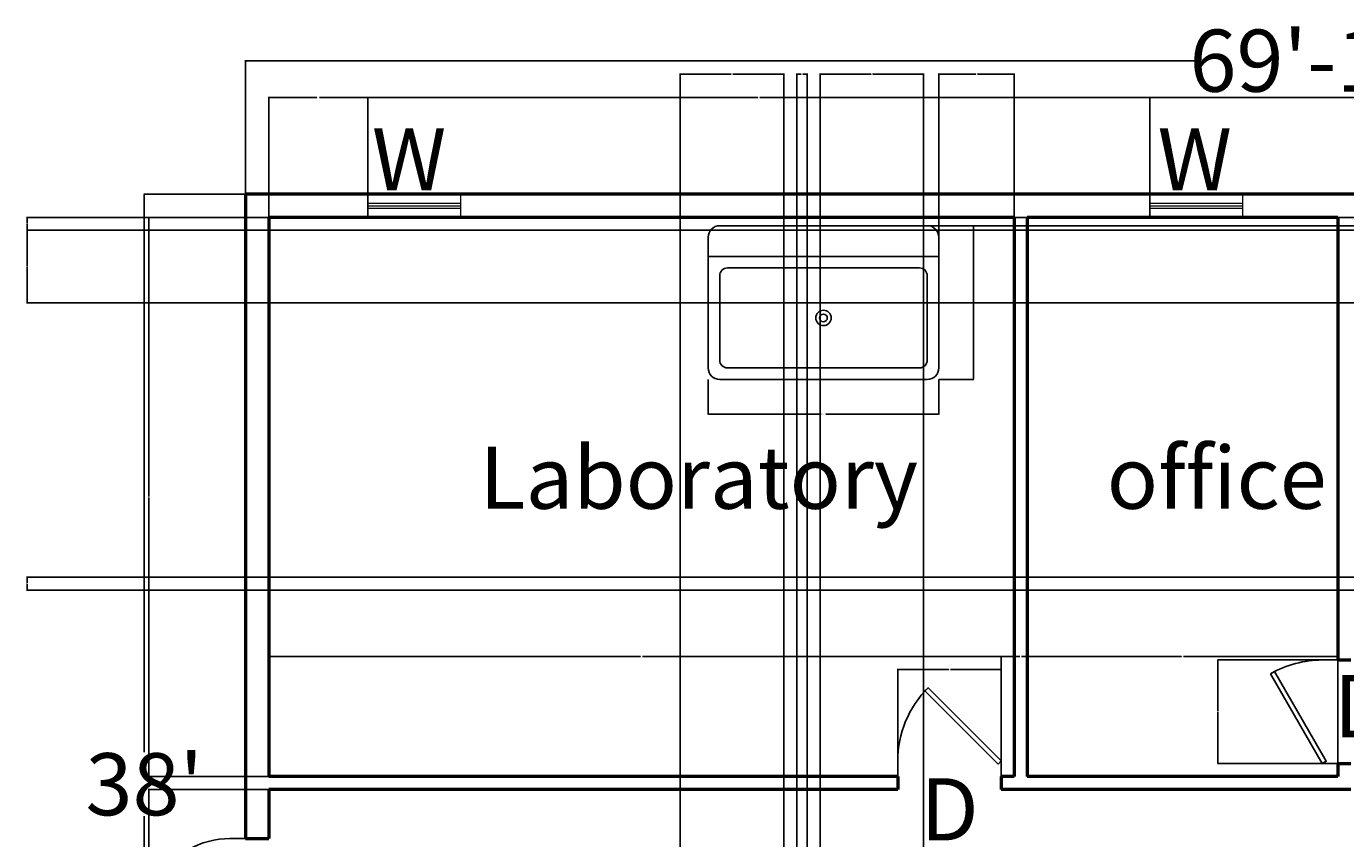
# Model space of a CAD drawing. Units: inches. Extents: x -84 to 931, y 65 to 668.
# Tile 2 of 5: x -84 to 426, y 355 to 668. Entities that reach past the tile are written whole.
import ezdxf

# ---------------------------------------------------------------- set-up
doc = ezdxf.new("R2010")
doc.units = ezdxf.units.IN
doc.header["$MEASUREMENT"] = 0
for name, color, linetype, lineweight in [('A-ANNO-DIMS', 2, 'Continuous', 18), ('A-ANNO-TEXT', 7, 'Continuous', 18), ('A-AREA-IDEN', 7, 'Continuous', 25), ('A-DOOR', 4, 'Continuous', 25), ('A-FLOR-FIXT', 9, 'Continuous', 25), ('A-GLAZ', 4, 'Continuous', 18), ('A-WALL', 7, 'Continuous', 50)]:
    doc.layers.add(name, color=color, linetype=linetype, lineweight=lineweight)
doc.styles.get("Standard").update_dxf_attribs({"font": 'arial.ttf'})
doc.dimstyles.get("Standard").update_dxf_attribs({"dimtxt": 0.18, "dimasz": 0.18, "dimexe": 0.18, "dimexo": 0.0625, "dimgap": 0.09, "dimtad": 0, "dimtih": 1, "dimtoh": 1, "dimdec": 0, "dimzin": 0, "dimdsep": 46, "dimlunit": 3, "dimtxsty": 'Standard', "dimcen": 0.09, "dimadec": 0, "dimazin": 0, "dimtfac": 1, "dimtdec": 0, "dimtofl": 0, "dimtmove": 0, "dimatfit": 3, "dimfxl": 1, "dimtolj": 1, "dimtzin": 0, "dimarcsym": 0})

# ---------------------------------------------------------------- blocks, each defined once
blk = doc.blocks.new('*U2')
for p, q in [((0, 0), (0, -6)), ((-40, 0), (-40, -6))]:
    blk.add_line(p, q)
blk.add_lwpolyline([(0, 0), (-28.28, 28.28), (-29.52, 27.05), (-1.24, -1.24)], close=True)
blk.add_arc((0, 0), 40, 135, 180)
blk = doc.blocks.new('*U3')
for p, q in [((0, 0), (0, -6)), ((40, 0), (40, -6))]:
    blk.add_line(p, q)
blk.add_lwpolyline([(0, 0), (34.64, 20), (35.52, 18.48), (0.88, -1.52)], close=True)
blk.add_arc((0, 0), 40, 0, 30)
blk = doc.blocks.new('*U11')
for p, q in [((0, 0), (0, -6)), ((32, 0), (32, -6))]:
    blk.add_line(p, q)
blk.add_lwpolyline([(0, 0), (27.71, 16), (28.59, 14.48), (0.87, -1.52)], close=True)
blk.add_arc((0, 0), 32, 0, 30)
blk = doc.blocks.new('Sink-single - 30 in top')
blk.add_line((-15, -3.999996), (15, -3.999996))
for points in [[(-13.5, 0), (13.5, 0)], [(-15, -18.499996), (-15, -1.5)], [(15, -1.5), (15, -18.499996)], [(-13.5, -17.499996), (-13.5, -6.499996)], [(-12.5, -5.499996), (12.5, -5.499996)], [(13.5, -6.499996), (13.5, -17.499996)], [(12.5, -18.499996), (-12.5, -18.499996)], [(13.5, -19.999996), (-13.5, -19.999996)]]:
    blk.add_lwpolyline(points)
for radius in [1, 0.5]:
    blk.add_circle((0, -11.999996), radius)
for centre, radius, start, end in [((-13.5, -1.5), 1.5, 90, 180), ((13.5, -1.5), 1.5, 0, 90), ((-12.5, -6.499996), 1, 90, 180), ((12.5, -6.499996), 1, 0, 90), ((-13.5, -18.499996), 1.5, 180, 270), ((-12.5, -17.499996), 1, 180, 270), ((12.5, -17.499996), 1, 270, 0), ((13.5, -18.499996), 1.5, 270, 0)]:
    blk.add_arc(centre, radius, start, end)
blk = doc.blocks.new('*D17')
at = {"layer": 'A-ANNO-DIMS', "color": 0, "lineweight": -2, "transparency": 16777216}
for p, q in [((0.53, 603.58), (0.53, 655.22)), ((0.71, 655.04), (368.83, 655.04)), ((838.35, 655.04), (470.23, 655.04)), ((838.53, 603.58), (838.53, 655.22))]:
    blk.add_line(p, q, dxfattribs=at)
at = {"layer": 'A-ANNO-DIMS', "color": 0, "transparency": 16777216}
for points in [[(0.71, 655.07), (0.71, 655.01), (0.53, 655.04)], [(838.35, 655.07), (838.35, 655.01), (838.53, 655.04)]]:
    blk.add_solid(points, dxfattribs=at)
at = {"layer": 'Defpoints', "color": 0, "transparency": 16777216}
for p in [(838.53, 655.04), (0.53, 603.52), (838.53, 603.52)]:
    blk.add_point(p, dxfattribs=at)
at = {"layer": 'A-ANNO-DIMS', "color": 0, "transparency": 16777216, "insert": (419.53, 655.04), "char_height": 0.18, "attachment_point": 5}
blk.add_mtext('\\A1;{\\H133.33333x;69\'-10"}', dxfattribs=at)
blk = doc.blocks.new('*D18')
at = {"layer": 'A-ANNO-DIMS', "color": 0, "lineweight": -2, "transparency": 16777216}
for p, q in [((0.47, 603.52), (-38.72, 603.52)), ((-38.54, 603.34), (-38.54, 387.87)), ((-38.54, 147.7), (-38.54, 363.16)), ((0.47, 147.52), (-38.72, 147.52))]:
    blk.add_line(p, q, dxfattribs=at)
at = {"layer": 'A-ANNO-DIMS', "color": 0, "transparency": 16777216}
for points in [[(-38.57, 603.34), (-38.51, 603.34), (-38.54, 603.52)], [(-38.57, 147.7), (-38.51, 147.7), (-38.54, 147.52)]]:
    blk.add_solid(points, dxfattribs=at)
at = {"layer": 'Defpoints', "color": 0, "transparency": 16777216}
for p in [(0.53, 603.52), (-38.54, 147.52), (0.53, 147.52)]:
    blk.add_point(p, dxfattribs=at)
at = {"layer": 'A-ANNO-DIMS', "color": 0, "transparency": 16777216, "insert": (-38.54, 375.52), "char_height": 0.18, "attachment_point": 5}
blk.add_mtext("\\A1;{\\H133.33333x;38'}", dxfattribs=at)
blk = doc.blocks.new('WIN-36IN')
for p, q in [((3.5, 0), (3.5, 36)), ((4.5, 0), (4.5, 36)), ((5.5, 0), (5.5, 36))]:
    blk.add_line(p, q)
blk.add_lwpolyline([(0, 36), (0, 0), (9, 0), (9, 36)], close=True)
blk = doc.blocks.new('*D29')
at = {"layer": 'A-ANNO-DIMS', "color": 0, "lineweight": -2, "transparency": 16777216}
for p, q in [((179.29, 531.84), (179.29, 518.36)), ((268.38, 531.84), (268.38, 518.36)), ((179.47, 518.54), (222.91, 518.54)), ((268.2, 518.54), (224.76, 518.54))]:
    blk.add_line(p, q, dxfattribs=at)
at = {"layer": 'A-ANNO-DIMS', "color": 0, "transparency": 16777216}
for points in [[(179.47, 518.57), (179.47, 518.51), (179.29, 518.54)], [(268.2, 518.57), (268.2, 518.51), (268.38, 518.54)]]:
    blk.add_solid(points, dxfattribs=at)
at = {"layer": 'Defpoints', "color": 0, "transparency": 16777216}
for p in [(179.29, 531.9), (268.38, 531.9), (268.38, 518.54)]:
    blk.add_point(p, dxfattribs=at)
at = {"layer": 'A-ANNO-DIMS', "color": 0, "transparency": 16777216, "insert": (223.83, 518.54), "char_height": 0.18, "attachment_point": 5}
blk.add_mtext('\\A1;LAB SINK 7\'-5"', dxfattribs=at)
blk = doc.blocks.new('*D30')
at = {"layer": 'A-ANNO-DIMS', "color": 0, "lineweight": -2, "transparency": 16777216}
for p, q in [((268.44, 591.29), (281.92, 591.29)), ((281.74, 591.11), (281.74, 561.78)), ((281.74, 532.08), (281.74, 561.42)), ((268.44, 531.9), (281.92, 531.9))]:
    blk.add_line(p, q, dxfattribs=at)
at = {"layer": 'A-ANNO-DIMS', "color": 0, "transparency": 16777216}
for points in [[(281.71, 591.11), (281.77, 591.11), (281.74, 591.29)], [(281.71, 532.08), (281.77, 532.08), (281.74, 531.9)]]:
    blk.add_solid(points, dxfattribs=at)
at = {"layer": 'Defpoints', "color": 0, "transparency": 16777216}
for p in [(268.38, 591.29), (281.74, 591.29), (268.38, 531.9)]:
    blk.add_point(p, dxfattribs=at)
at = {"layer": 'A-ANNO-DIMS', "color": 0, "transparency": 16777216, "insert": (281.74, 561.6), "char_height": 0.18, "attachment_point": 5}
blk.add_mtext('\\A1;4\'-11 1/2"', dxfattribs=at)
blk = doc.blocks.new('*D33')
at = {"layer": 'A-ANNO-DIMS', "color": 0, "lineweight": -2, "transparency": 16777216}
for p, q in [((9.53, 594.58), (9.53, 641.05)), ((9.71, 640.87), (28.12, 640.87)), ((47.62, 640.87), (29.2, 640.87)), ((47.8, 594.58), (47.8, 641.05))]:
    blk.add_line(p, q, dxfattribs=at)
at = {"layer": 'A-ANNO-DIMS', "color": 0, "transparency": 16777216}
for points in [[(9.71, 640.9), (9.71, 640.84), (9.53, 640.87)], [(47.62, 640.9), (47.62, 640.84), (47.8, 640.87)]]:
    blk.add_solid(points, dxfattribs=at)
at = {"layer": 'Defpoints', "color": 0, "transparency": 16777216}
for p in [(47.8, 640.87), (9.53, 594.52), (47.8, 594.52)]:
    blk.add_point(p, dxfattribs=at)
at = {"layer": 'A-ANNO-DIMS', "color": 0, "transparency": 16777216, "insert": (28.66, 640.87), "char_height": 0.18, "attachment_point": 5}
blk.add_mtext('\\A1;3\'-2 1/2"', dxfattribs=at)
blk = doc.blocks.new('*D34')
at = {"layer": 'A-ANNO-DIMS', "color": 0, "lineweight": -2, "transparency": 16777216}
for p, q in [((47.8, 594.58), (47.8, 641.05)), ((47.98, 640.87), (198.42, 640.87)), ((349.67, 640.87), (199.22, 640.87)), ((349.85, 594.58), (349.85, 641.05))]:
    blk.add_line(p, q, dxfattribs=at)
at = {"layer": 'A-ANNO-DIMS', "color": 0, "transparency": 16777216}
for points in [[(47.98, 640.9), (47.98, 640.84), (47.8, 640.87)], [(349.67, 640.9), (349.67, 640.84), (349.85, 640.87)]]:
    blk.add_solid(points, dxfattribs=at)
at = {"layer": 'Defpoints', "color": 0, "transparency": 16777216}
for p in [(349.85, 640.87), (47.8, 594.52), (349.85, 594.52)]:
    blk.add_point(p, dxfattribs=at)
at = {"layer": 'A-ANNO-DIMS', "color": 0, "transparency": 16777216, "insert": (198.82, 640.87), "char_height": 0.18, "attachment_point": 5}
blk.add_mtext('\\A1;25\'-2"', dxfattribs=at)
blk = doc.blocks.new('*D35')
at = {"layer": 'A-ANNO-DIMS', "color": 0, "lineweight": -2, "transparency": 16777216}
for p, q in [((349.85, 594.58), (349.85, 641.05)), ((350.03, 640.87), (444.4, 640.87)), ((539.69, 640.87), (445.32, 640.87)), ((539.87, 594.58), (539.87, 641.05))]:
    blk.add_line(p, q, dxfattribs=at)
at = {"layer": 'A-ANNO-DIMS', "color": 0, "transparency": 16777216}
for points in [[(350.03, 640.9), (350.03, 640.84), (349.85, 640.87)], [(539.69, 640.9), (539.69, 640.84), (539.87, 640.87)]]:
    blk.add_solid(points, dxfattribs=at)
at = {"layer": 'Defpoints', "color": 0, "transparency": 16777216}
for p in [(539.87, 640.87), (349.85, 594.52), (539.87, 594.52)]:
    blk.add_point(p, dxfattribs=at)
at = {"layer": 'A-ANNO-DIMS', "color": 0, "transparency": 16777216, "insert": (444.86, 640.87), "char_height": 0.18, "attachment_point": 5}
blk.add_mtext('\\A1;15\'-10"', dxfattribs=at)
blk = doc.blocks.new('*D36')
at = {"layer": 'A-ANNO-DIMS', "color": 0, "lineweight": -2, "transparency": 16777216}
for p, q in [((9.53, 378.58), (9.53, 425.05)), ((9.71, 424.87), (153.13, 424.87)), ((297.35, 424.87), (153.93, 424.87)), ((297.53, 378.58), (297.53, 425.05))]:
    blk.add_line(p, q, dxfattribs=at)
at = {"layer": 'A-ANNO-DIMS', "color": 0, "transparency": 16777216}
for points in [[(9.71, 424.9), (9.71, 424.84), (9.53, 424.87)], [(297.35, 424.9), (297.35, 424.84), (297.53, 424.87)]]:
    blk.add_solid(points, dxfattribs=at)
at = {"layer": 'Defpoints', "color": 0, "transparency": 16777216}
for p in [(297.53, 424.87), (9.53, 378.52), (297.53, 378.52)]:
    blk.add_point(p, dxfattribs=at)
at = {"layer": 'A-ANNO-DIMS', "color": 0, "transparency": 16777216, "insert": (153.53, 424.87), "char_height": 0.18, "attachment_point": 5}
blk.add_mtext('\\A1;24\'-0"', dxfattribs=at)
blk = doc.blocks.new('*D37')
at = {"layer": 'A-ANNO-DIMS', "color": 0, "lineweight": -2, "transparency": 16777216}
for p, q in [((302.53, 378.58), (302.53, 425.05)), ((302.71, 424.87), (362.14, 424.87)), ((422.35, 424.87), (362.92, 424.87)), ((422.53, 378.58), (422.53, 425.05))]:
    blk.add_line(p, q, dxfattribs=at)
at = {"layer": 'A-ANNO-DIMS', "color": 0, "transparency": 16777216}
for points in [[(302.71, 424.9), (302.71, 424.84), (302.53, 424.87)], [(422.35, 424.9), (422.35, 424.84), (422.53, 424.87)]]:
    blk.add_solid(points, dxfattribs=at)
at = {"layer": 'Defpoints', "color": 0, "transparency": 16777216}
for p in [(422.53, 424.87), (302.53, 378.52), (422.53, 378.52)]:
    blk.add_point(p, dxfattribs=at)
at = {"layer": 'A-ANNO-DIMS', "color": 0, "transparency": 16777216, "insert": (362.53, 424.87), "char_height": 0.18, "attachment_point": 5}
blk.add_mtext('\\A1;10\'-0"', dxfattribs=at)
blk = doc.blocks.new('*D46')
at = {"layer": 'A-ANNO-DIMS', "color": 0, "lineweight": -2, "transparency": 16777216}
for p, q in [((9.47, 594.52), (-37, 594.52)), ((-36.82, 594.34), (-36.82, 486.7)), ((-36.82, 378.7), (-36.82, 486.33)), ((9.47, 378.52), (-37, 378.52))]:
    blk.add_line(p, q, dxfattribs=at)
at = {"layer": 'A-ANNO-DIMS', "color": 0, "transparency": 16777216}
for points in [[(-36.85, 594.34), (-36.79, 594.34), (-36.82, 594.52)], [(-36.85, 378.7), (-36.79, 378.7), (-36.82, 378.52)]]:
    blk.add_solid(points, dxfattribs=at)
at = {"layer": 'Defpoints', "color": 0, "transparency": 16777216}
for p in [(-36.82, 594.52), (9.53, 594.52), (9.53, 378.52)]:
    blk.add_point(p, dxfattribs=at)
at = {"layer": 'A-ANNO-DIMS', "color": 0, "transparency": 16777216, "insert": (-36.82, 486.52), "char_height": 0.18, "attachment_point": 5}
blk.add_mtext('\\A1;18\'-0"', dxfattribs=at)
blk = doc.blocks.new('*D47')
at = {"layer": 'A-ANNO-DIMS', "color": 0, "lineweight": -2, "transparency": 16777216}
for p, q in [((9.47, 373.52), (-37, 373.52)), ((-36.82, 373.34), (-36.82, 345.7)), ((-36.82, 317.7), (-36.82, 345.33)), ((9.47, 317.52), (-37, 317.52))]:
    blk.add_line(p, q, dxfattribs=at)
at = {"layer": 'A-ANNO-DIMS', "color": 0, "transparency": 16777216}
for points in [[(-36.85, 373.34), (-36.79, 373.34), (-36.82, 373.52)], [(-36.85, 317.7), (-36.79, 317.7), (-36.82, 317.52)]]:
    blk.add_solid(points, dxfattribs=at)
at = {"layer": 'Defpoints', "color": 0, "transparency": 16777216}
for p in [(-36.82, 373.52), (9.53, 373.52), (9.53, 317.52)]:
    blk.add_point(p, dxfattribs=at)
at = {"layer": 'A-ANNO-DIMS', "color": 0, "transparency": 16777216, "insert": (-36.82, 345.52), "char_height": 0.18, "attachment_point": 5}
blk.add_mtext('\\A1;4\'-8"', dxfattribs=at)
blk = doc.blocks.new('*D54')
at = {"layer": 'A-ANNO-DIMS', "color": 0, "lineweight": -2, "transparency": 16777216}
for p, q in [((252.53, 373.58), (252.53, 420.05)), ((252.71, 419.87), (272.2, 419.87)), ((292.35, 419.87), (272.86, 419.87)), ((292.53, 373.58), (292.53, 420.05))]:
    blk.add_line(p, q, dxfattribs=at)
at = {"layer": 'A-ANNO-DIMS', "color": 0, "transparency": 16777216}
for points in [[(252.71, 419.9), (252.71, 419.84), (252.53, 419.87)], [(292.35, 419.9), (292.35, 419.84), (292.53, 419.87)]]:
    blk.add_solid(points, dxfattribs=at)
at = {"layer": 'Defpoints', "color": 0, "transparency": 16777216}
for p in [(292.53, 419.87), (252.53, 373.52), (292.53, 373.52)]:
    blk.add_point(p, dxfattribs=at)
at = {"layer": 'A-ANNO-DIMS', "color": 0, "transparency": 16777216, "insert": (272.53, 419.87), "char_height": 0.18, "attachment_point": 5}
blk.add_mtext('\\A1;3\'-4"', dxfattribs=at)
blk = doc.blocks.new('*D55')
at = {"layer": 'A-ANNO-DIMS', "color": 0, "lineweight": -2, "transparency": 16777216}
for p, q in [((704.47, 589.52), (-84, 589.52)), ((-83.82, 589.34), (-83.82, 575.7)), ((-83.82, 561.7), (-83.82, 575.34)), ((704.47, 561.52), (-84, 561.52))]:
    blk.add_line(p, q, dxfattribs=at)
at = {"layer": 'A-ANNO-DIMS', "color": 0, "transparency": 16777216}
for points in [[(-83.85, 589.34), (-83.79, 589.34), (-83.82, 589.52)], [(-83.85, 561.7), (-83.79, 561.7), (-83.82, 561.52)]]:
    blk.add_solid(points, dxfattribs=at)
at = {"layer": 'Defpoints', "color": 0, "transparency": 16777216}
for p in [(-83.82, 589.52), (704.53, 589.52), (704.53, 561.52)]:
    blk.add_point(p, dxfattribs=at)
at = {"layer": 'A-ANNO-DIMS', "color": 0, "transparency": 16777216, "insert": (-83.82, 575.52), "char_height": 0.18, "attachment_point": 5}
blk.add_mtext('\\A1;2\'-4"', dxfattribs=at)
blk = doc.blocks.new('*D69')
at = {"layer": 'A-ANNO-DIMS', "color": 0, "lineweight": -2, "transparency": 16777216}
for p, q in [((168.52, 312.58), (168.52, 650.05)), ((168.7, 649.87), (188.2, 649.87)), ((208.35, 649.87), (188.86, 649.87)), ((208.53, 312.58), (208.53, 650.05))]:
    blk.add_line(p, q, dxfattribs=at)
at = {"layer": 'A-ANNO-DIMS', "color": 0, "transparency": 16777216}
for points in [[(168.7, 649.9), (168.7, 649.84), (168.52, 649.87)], [(208.35, 649.9), (208.35, 649.84), (208.53, 649.87)]]:
    blk.add_solid(points, dxfattribs=at)
at = {"layer": 'Defpoints', "color": 0, "transparency": 16777216}
for p in [(208.53, 649.87), (168.52, 312.52), (208.53, 312.52)]:
    blk.add_point(p, dxfattribs=at)
at = {"layer": 'A-ANNO-DIMS', "color": 0, "transparency": 16777216, "insert": (188.53, 649.87), "char_height": 0.18, "attachment_point": 5}
blk.add_mtext('\\A1;3\'-4"', dxfattribs=at)
blk = doc.blocks.new('*D70')
at = {"layer": 'A-ANNO-DIMS', "color": 0, "lineweight": -2, "transparency": 16777216}
for p, q in [((222.53, 312.58), (222.53, 650.05)), ((222.71, 649.87), (242.2, 649.87)), ((262.35, 649.87), (242.86, 649.87)), ((262.53, 312.58), (262.53, 650.05))]:
    blk.add_line(p, q, dxfattribs=at)
at = {"layer": 'A-ANNO-DIMS', "color": 0, "transparency": 16777216}
for points in [[(222.71, 649.9), (222.71, 649.84), (222.53, 649.87)], [(262.35, 649.9), (262.35, 649.84), (262.53, 649.87)]]:
    blk.add_solid(points, dxfattribs=at)
at = {"layer": 'Defpoints', "color": 0, "transparency": 16777216}
for p in [(262.53, 649.87), (222.53, 312.52), (262.53, 312.52)]:
    blk.add_point(p, dxfattribs=at)
at = {"layer": 'A-ANNO-DIMS', "color": 0, "transparency": 16777216, "insert": (242.53, 649.87), "char_height": 0.18, "attachment_point": 5}
blk.add_mtext('\\A1;3\'-4"', dxfattribs=at)
blk = doc.blocks.new('*D73')
at = {"layer": 'A-ANNO-DIMS', "color": 0, "lineweight": -2, "transparency": 16777216}
for p, q in [((213.53, 156.58), (213.53, 650.05)), ((213.71, 649.87), (215.2, 649.87)), ((217.35, 649.87), (215.86, 649.87)), ((217.53, 156.58), (217.53, 650.05))]:
    blk.add_line(p, q, dxfattribs=at)
at = {"layer": 'A-ANNO-DIMS', "color": 0, "transparency": 16777216}
for points in [[(213.71, 649.9), (213.71, 649.84), (213.53, 649.87)], [(217.35, 649.9), (217.35, 649.84), (217.53, 649.87)]]:
    blk.add_solid(points, dxfattribs=at)
at = {"layer": 'Defpoints', "color": 0, "transparency": 16777216}
for p in [(217.53, 649.87), (213.53, 156.52), (217.53, 156.52)]:
    blk.add_point(p, dxfattribs=at)
at = {"layer": 'A-ANNO-DIMS', "color": 0, "transparency": 16777216, "insert": (215.53, 649.87), "char_height": 0.18, "attachment_point": 5}
blk.add_mtext('\\A1;0\'-4"', dxfattribs=at)
blk = doc.blocks.new('*D74')
at = {"layer": 'A-ANNO-DIMS', "color": 0, "lineweight": -2, "transparency": 16777216}
for p, q in [((297.53, 378.58), (297.53, 425.05)), ((297.71, 424.87), (299.7, 424.87)), ((302.35, 424.87), (300.36, 424.87)), ((302.53, 378.58), (302.53, 425.05))]:
    blk.add_line(p, q, dxfattribs=at)
at = {"layer": 'A-ANNO-DIMS', "color": 0, "transparency": 16777216}
for points in [[(297.71, 424.9), (297.71, 424.84), (297.53, 424.87)], [(302.35, 424.9), (302.35, 424.84), (302.53, 424.87)]]:
    blk.add_solid(points, dxfattribs=at)
at = {"layer": 'Defpoints', "color": 0, "transparency": 16777216}
for p in [(302.53, 424.87), (297.53, 378.52), (302.53, 378.52)]:
    blk.add_point(p, dxfattribs=at)
at = {"layer": 'A-ANNO-DIMS', "color": 0, "transparency": 16777216, "insert": (300.03, 424.87), "char_height": 0.18, "attachment_point": 5}
blk.add_mtext('\\A1;0\'-5"', dxfattribs=at)
blk = doc.blocks.new('*D75')
at = {"layer": 'A-ANNO-DIMS', "color": 0, "lineweight": -2, "transparency": 16777216}
for p, q in [((268.38, 586.9), (268.38, 650.05)), ((268.56, 649.87), (282.62, 649.87)), ((297.35, 649.87), (283.28, 649.87)), ((297.53, 594.58), (297.53, 650.05))]:
    blk.add_line(p, q, dxfattribs=at)
at = {"layer": 'A-ANNO-DIMS', "color": 0, "transparency": 16777216}
for points in [[(268.56, 649.9), (268.56, 649.84), (268.38, 649.87)], [(297.35, 649.9), (297.35, 649.84), (297.53, 649.87)]]:
    blk.add_solid(points, dxfattribs=at)
at = {"layer": 'Defpoints', "color": 0, "transparency": 16777216}
for p in [(297.53, 649.87), (297.53, 594.52), (268.38, 586.84)]:
    blk.add_point(p, dxfattribs=at)
at = {"layer": 'A-ANNO-DIMS', "color": 0, "transparency": 16777216, "insert": (282.95, 649.87), "char_height": 0.18, "attachment_point": 5}
blk.add_mtext('\\A1;2\'-5"', dxfattribs=at)
blk = doc.blocks.new('*D76')
at = {"layer": 'A-ANNO-DIMS', "color": 0, "lineweight": -2, "transparency": 16777216}
for p, q in [((263.98, 591.29), (931.06, 591.29)), ((297.59, 594.52), (931.06, 594.52)), ((930.88, 594.34), (930.88, 593.09)), ((930.88, 591.47), (930.88, 592.72))]:
    blk.add_line(p, q, dxfattribs=at)
at = {"layer": 'A-ANNO-DIMS', "color": 0, "transparency": 16777216}
for points in [[(930.85, 594.34), (930.91, 594.34), (930.88, 594.52)], [(930.85, 591.47), (930.91, 591.47), (930.88, 591.29)]]:
    blk.add_solid(points, dxfattribs=at)
at = {"layer": 'Defpoints', "color": 0, "transparency": 16777216}
for p in [(263.92, 591.29), (297.53, 594.52), (930.88, 594.52)]:
    blk.add_point(p, dxfattribs=at)
at = {"layer": 'A-ANNO-DIMS', "color": 0, "transparency": 16777216, "insert": (930.88, 592.9), "char_height": 0.18, "attachment_point": 5}
blk.add_mtext('\\A1;0\'-3"', dxfattribs=at)
blk = doc.blocks.new('*D83')
at = {"layer": 'A-ANNO-DIMS', "color": 0, "lineweight": -2, "transparency": 16777216}
for p, q in [((709.47, 594.52), (-84, 594.52)), ((-83.82, 594.34), (-83.82, 592.2)), ((-83.82, 589.7), (-83.82, 591.83)), ((709.47, 589.52), (-84, 589.52))]:
    blk.add_line(p, q, dxfattribs=at)
at = {"layer": 'A-ANNO-DIMS', "color": 0, "transparency": 16777216}
for points in [[(-83.85, 594.34), (-83.79, 594.34), (-83.82, 594.52)], [(-83.85, 589.7), (-83.79, 589.7), (-83.82, 589.52)]]:
    blk.add_solid(points, dxfattribs=at)
at = {"layer": 'Defpoints', "color": 0, "transparency": 16777216}
for p in [(-83.82, 594.52), (709.53, 594.52), (709.53, 589.52)]:
    blk.add_point(p, dxfattribs=at)
at = {"layer": 'A-ANNO-DIMS', "color": 0, "transparency": 16777216, "insert": (-83.82, 592.02), "char_height": 0.18, "attachment_point": 5}
blk.add_mtext('\\A1;0\'-5"', dxfattribs=at)
blk = doc.blocks.new('*D84')
at = {"layer": 'A-ANNO-DIMS', "color": 0, "lineweight": -2, "transparency": 16777216}
for p, q in [((709.47, 455.52), (-84, 455.52)), ((-83.82, 455.34), (-83.82, 453.2)), ((709.47, 450.52), (-84, 450.52)), ((-83.82, 450.7), (-83.82, 452.83))]:
    blk.add_line(p, q, dxfattribs=at)
at = {"layer": 'A-ANNO-DIMS', "color": 0, "transparency": 16777216}
for points in [[(-83.85, 455.34), (-83.79, 455.34), (-83.82, 455.52)], [(-83.85, 450.7), (-83.79, 450.7), (-83.82, 450.52)]]:
    blk.add_solid(points, dxfattribs=at)
at = {"layer": 'Defpoints', "color": 0, "transparency": 16777216}
for p in [(709.53, 455.52), (-83.82, 450.52), (709.53, 450.52)]:
    blk.add_point(p, dxfattribs=at)
at = {"layer": 'A-ANNO-DIMS', "color": 0, "transparency": 16777216, "insert": (-83.82, 453.02), "char_height": 0.18, "attachment_point": 5}
blk.add_mtext('\\A1;0\'-5"', dxfattribs=at)
blk = doc.blocks.new('*D85')
at = {"layer": 'A-ANNO-DIMS', "color": 0, "lineweight": -2, "transparency": 16777216}
for p, q in [((422.47, 423.52), (376, 423.52)), ((376.18, 423.34), (376.18, 403.7)), ((376.18, 383.7), (376.18, 403.33)), ((422.47, 383.52), (376, 383.52))]:
    blk.add_line(p, q, dxfattribs=at)
at = {"layer": 'A-ANNO-DIMS', "color": 0, "transparency": 16777216}
for points in [[(376.15, 423.34), (376.21, 423.34), (376.18, 423.52)], [(376.15, 383.7), (376.21, 383.7), (376.18, 383.52)]]:
    blk.add_solid(points, dxfattribs=at)
at = {"layer": 'Defpoints', "color": 0, "transparency": 16777216}
for p in [(376.18, 423.52), (422.53, 423.52), (422.53, 383.52)]:
    blk.add_point(p, dxfattribs=at)
at = {"layer": 'A-ANNO-DIMS', "color": 0, "transparency": 16777216, "insert": (376.18, 403.52), "char_height": 0.18, "attachment_point": 5}
blk.add_mtext('\\A1;3\'-4"', dxfattribs=at)
blk = doc.blocks.new('*D88')
at = {"layer": 'A-ANNO-DIMS', "color": 0, "lineweight": -2, "transparency": 16777216}
for p, q in [((292.53, 378.58), (292.53, 425.05)), ((292.71, 424.87), (294.7, 424.87)), ((297.35, 424.87), (295.36, 424.87)), ((297.53, 378.58), (297.53, 425.05))]:
    blk.add_line(p, q, dxfattribs=at)
at = {"layer": 'A-ANNO-DIMS', "color": 0, "transparency": 16777216}
for points in [[(292.71, 424.9), (292.71, 424.84), (292.53, 424.87)], [(297.35, 424.9), (297.35, 424.84), (297.53, 424.87)]]:
    blk.add_solid(points, dxfattribs=at)
at = {"layer": 'Defpoints', "color": 0, "transparency": 16777216}
for p in [(297.53, 424.87), (292.53, 378.52), (297.53, 378.52)]:
    blk.add_point(p, dxfattribs=at)
at = {"layer": 'A-ANNO-DIMS', "color": 0, "transparency": 16777216, "insert": (295.03, 424.87), "char_height": 0.18, "attachment_point": 5}
blk.add_mtext('\\A1;0\'-5"', dxfattribs=at)

msp = doc.modelspace()

# ---------------------------------------------------------------- linework, layer by layer
at = {"layer": 'A-WALL'}
for p, q in [((672.53, 603.52), (0.53, 603.52)), ((0.53, 603.52), (0.53, 354.52)), ((9.53, 594.52), (9.53, 378.52)), ((297.53, 594.52), (9.53, 594.52)), ((297.53, 594.52), (297.53, 378.52)), ((302.53, 594.52), (302.53, 378.52)), ((422.53, 594.52), (302.53, 594.52)), ((422.53, 594.52), (422.53, 423.52)), ((422.53, 423.52), (427.53, 423.52)), ((422.53, 383.52), (427.53, 383.52)), ((422.53, 383.52), (422.53, 378.52)), ((252.53, 378.52), (9.53, 378.52)), ((252.53, 378.52), (252.53, 373.52)), ((297.53, 378.52), (292.53, 378.52)), ((292.53, 378.52), (292.53, 373.52)), ((422.53, 378.52), (302.53, 378.52)), ((9.53, 373.52), (9.53, 354.52)), ((252.53, 373.52), (9.53, 373.52)), ((427.53, 373.52), (292.53, 373.52)), ((0.53, 354.52), (9.53, 354.52))]:
    msp.add_line(p, q, dxfattribs=at)

# ---------------------------------------------------------------- block references
at = {"layer": 'A-DOOR', "rotation": 90}
for name, p in [('*U3', (416.53, 383.52)), ('*U11', (-5.47, 322.52))]:
    msp.add_blockref(name, p, dxfattribs=at)
at = {"layer": 'A-DOOR'}
msp.add_blockref('*U2', (292.53, 384.52), dxfattribs=at)
at = {"layer": 'A-FLOR-FIXT', "xscale": 2.969465553422717, "yscale": 2.969465553422717, "zscale": 2.969465553422717}
msp.add_blockref('Sink-single - 30 in top', (223.83, 591.29), dxfattribs=at)
at = {"layer": 'A-GLAZ', "rotation": 269.9999999999999}
for p in [(47.8, 603.52), (349.85, 603.52)]:
    msp.add_blockref('WIN-36IN', p, dxfattribs=at)

# ---------------------------------------------------------------- texts
at = {"layer": 'A-ANNO-TEXT', "char_height": 24, "attachment_point": 1}
for s, width, insert in [('W', 20.4711, (49.37, 628.94)), ('W', 20.4711, (352.87, 628.94)), ('D', 21.9508, (420.9, 417.69)), ('D', 21.9508, (261.26, 377.82))]:
    msp.add_mtext_dynamic_manual_height_columns(s, width=width, gutter_width=1, heights=[0], dxfattribs=dict(at, insert=insert))
at = {"layer": 'A-AREA-IDEN', "char_height": 24, "attachment_point": 1}
for s, width, insert in [('Laboratory', 108.66, (90.97, 505.94)), ('office', 70.4822, (333.25, 505.94))]:
    msp.add_mtext_dynamic_manual_height_columns(s, width=width, gutter_width=1, heights=[0], dxfattribs=dict(at, insert=insert))

# ---------------------------------------------------------------- dimensions: what is measured, and where the dimension line sits
at = {"layer": 'A-ANNO-DIMS'}
for base, p1, p2, text, override, picture, middle in [((838.53, 655.04), (0.53, 603.52), (838.53, 603.52), '{\\H133.33333x;<>}', {"dimclrd": 0, "dimclre": 0, "dimclrt": 0}, '*D17', (419.53, 655.04)), ((268.38, 518.54), (179.29, 531.9), (268.38, 531.9), 'LAB SINK <>', {"dimdec": 1, "dimlfac": 1, "dimrnd": 0, "dimzin": 1, "dimdsep": 46, "dimlunit": 4, "dimfrac": 2}, '*D29', (223.83, 518.54))]:
    dim = msp.add_linear_dim(base=base, p1=p1, p2=p2, text=text, dimstyle='Standard', override=override, dxfattribs=at)
    dim.commit()
    dim.dimension.update_dxf_attribs({"geometry": picture, "text_midpoint": middle})
for base, p1, p2, picture, middle in [((208.53, 649.87), (168.52, 312.52), (208.53, 312.52), '*D69', (188.53, 649.87)), ((217.53, 649.87), (213.53, 156.52), (217.53, 156.52), '*D73', (215.53, 649.87)), ((262.53, 649.87), (222.53, 312.52), (262.53, 312.52), '*D70', (242.53, 649.87)), ((297.5304, 649.8657), (268.3765, 586.8394), (297.5304, 594.5157), '*D75', (282.9534, 649.8657)), ((47.8, 640.87), (9.53, 594.52), (47.8, 594.52), '*D33', (28.66, 640.87)), ((349.8485, 640.8657), (47.7961, 594.5157), (349.8485, 594.5157), '*D34', (198.8223, 640.8657)), ((539.87, 640.87), (349.85, 594.52), (539.87, 594.52), '*D35', (444.86, 640.87)), ((297.53, 424.87), (292.53, 378.52), (297.53, 378.52), '*D88', (295.03, 424.87)), ((302.53, 424.87), (297.53, 378.52), (302.53, 378.52), '*D74', (300.03, 424.87)), ((422.53, 424.87), (302.53, 378.52), (422.53, 378.52), '*D37', (362.53, 424.87)), ((292.53, 419.87), (252.53, 373.52), (292.53, 373.52), '*D54', (272.53, 419.87))]:
    dim = msp.add_linear_dim(base=base, p1=p1, p2=p2, dimstyle='Standard', override={"dimdec": 1, "dimlfac": 1, "dimrnd": 0, "dimzin": 1, "dimdsep": 46, "dimlunit": 4, "dimfrac": 2}, dxfattribs=at)
    dim.commit()
    dim.dimension.update_dxf_attribs({"geometry": picture, "text_midpoint": middle})
dim = msp.add_linear_dim(base=(-38.54, 147.52), p1=(0.53, 603.52), p2=(0.53, 147.52), angle=90, text='{\\H133.33333x;<>}', dimstyle='Standard', override={"dimclrd": 0, "dimclre": 0, "dimclrt": 0}, dxfattribs=at)
dim.commit()
dim.dimension.update_dxf_attribs({"geometry": '*D18', "text_midpoint": (-38.54, 375.52)})
for base, p1, p2, angle, picture, middle in [((-83.82, 594.52), (709.53, 589.52), (709.53, 594.52), 90, '*D83', (-83.82, 592.02)), ((-36.82, 594.52), (9.53, 378.52), (9.53, 594.52), 90, '*D46', (-36.82, 486.52)), ((930.88, 594.52), (263.92, 591.29), (297.53, 594.52), 90, '*D76', (930.88, 592.9)), ((281.74, 591.29), (268.38, 531.9), (268.38, 591.29), 90, '*D30', (281.74, 561.6)), ((-83.82, 589.52), (704.53, 561.52), (704.53, 589.52), 90, '*D55', (-83.82, 575.52)), ((-83.82, 450.52), (709.53, 455.52), (709.53, 450.52), 90, '*D84', (-83.82, 453.02)), ((297.53, 424.87), (9.53, 378.52), (297.53, 378.52), 0, '*D36', (153.53, 424.87)), ((376.18, 423.52), (422.53, 383.52), (422.53, 423.52), 90, '*D85', (376.18, 403.52)), ((-36.82, 373.52), (9.53, 317.52), (9.53, 373.52), 90, '*D47', (-36.82, 345.52))]:
    dim = msp.add_linear_dim(base=base, p1=p1, p2=p2, angle=angle, dimstyle='Standard', override={"dimdec": 1, "dimlfac": 1, "dimrnd": 0, "dimzin": 1, "dimdsep": 46, "dimlunit": 4, "dimfrac": 2}, dxfattribs=at)
    dim.commit()
    dim.dimension.update_dxf_attribs({"geometry": picture, "text_midpoint": middle})

doc.saveas('drawing.dxf')
